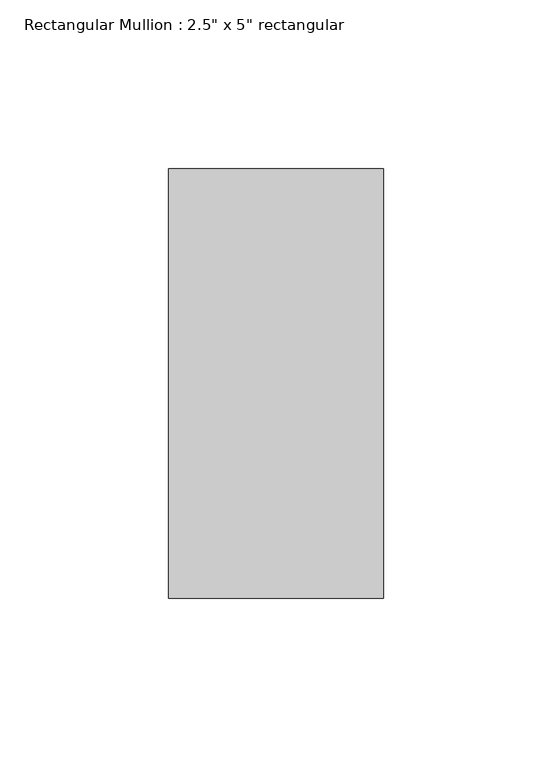
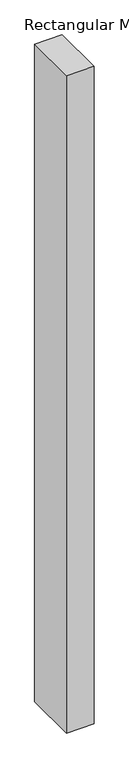
"""IFC4 building model written with IfcOpenShell, lengths in millimetres: member geometry."""

from ifc_helpers import new_model, si_unit, frame, origin, place, context, project, spatial, polyline, outline, extrude, source, transform, mapped, element, save


def member_8dd5f4d9(model_context):
    return source(origin(), model_context, "Body", "SweptSolid", [
        extrude(outline(polyline([(0.0, 63.5), (0.0, -63.5), (-63.5, -63.5), (-63.5, 63.5), (0.0, 63.5)])), frame((0.0, 0.0, -1605.5835026), z_axis=(0.0, 0.0, 1.0), x_axis=(1.0, 0.0, 0.0)), (0.0, 0.0, 1.0), 1605.5835026),
    ])


if __name__ == "__main__":
    model = new_model("IFC4")
    model_context = context("Model", 3, world=origin())
    ifc_project = project(units=[si_unit("LENGTHUNIT", "METRE", prefix="MILLI")], contexts=[model_context])
    site = spatial("IfcSite", under=ifc_project)
    building = spatial("IfcBuilding", under=site)
    placement = place(None, origin())
    member_shape = member_8dd5f4d9(model_context)
    element("IfcMember", 1, ObjectType="Rectangular Mullion : 2.5\" x 5\" rectangular", at=placement, inside=building, context=model_context, shape_type="MappedRepresentation", body=[
        mapped(member_shape, transform((0.0, 0.0, 0.0), x_axis=(1.0, 0.0, 0.0), y_axis=(0.0, 1.0, 0.0), z_axis=(0.0, 0.0, 1.0))),
    ])
    save(model, "model.ifc")

# Revit data of these elements
# Type "Rectangular Mullion : 2.5\" x 5\" rectangular"
#   built-in parameter 1007304 = 0.416667 (stored number, unit not read)
#   built-in parameter 1007301 = 0.104167 (stored number, unit not read)
#   built-in parameter 1007300 = 0.104167 (stored number, unit not read)
# Element 1 (IfcMember, "Rectangular Mullion : 2.5\" x 5\" rectangular")
#   Materials on its faces: "Aluminum"
# Materials
#   "Aluminum": class "Metal", colour RGB 247 247 247, transparency 0, Description = "Aluminum 6061", Cost = 0
